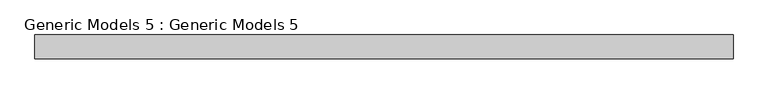
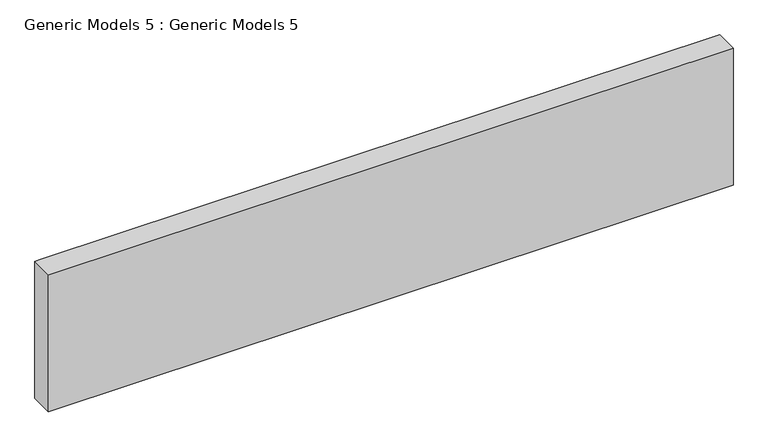
"""IFC4 building model written with IfcOpenShell, lengths in millimetres: proxy geometry, Generic Models 5 : Generic Models 5."""

from ifc_helpers import new_model, si_unit, origin, place, context, project, spatial, faceted_brep, source, transform, mapped, element, save


def generic_models_5_generic_models_5_9fe8e222(model_context):
    return source(origin(), model_context, "Body", "Brep", [
        faceted_brep([(-8586.8607234, -14006.5538163, 10395.767225), (-13013.8422243, -14006.5538163, 10395.767225), (-13059.291855, -14006.5538163, 10395.767225), (-13059.291855, -14158.9538163, 10395.767225), (-8586.8607234, -14158.9538163, 10395.767225), (-8586.8607234, -14006.5538163, 9448.8), (-8586.8607234, -14158.9538163, 9448.8), (-13059.291855, -14158.9538163, 9448.8), (-13059.291855, -14006.5538163, 9448.8), (-13013.8422243, -14006.5538163, 9448.8)], [[[0, 1, 2, 3, 4]], [[5, 6, 7, 8, 9]], [[2, 1, 0, 5, 9, 8]], [[3, 2, 8, 7]], [[4, 3, 7, 6]], [[0, 4, 6, 5]]]),
    ])


if __name__ == "__main__":
    model = new_model("IFC4")
    model_context = context("Model", 3, world=origin())
    ifc_project = project(units=[si_unit("LENGTHUNIT", "METRE", prefix="MILLI")], contexts=[model_context])
    site = spatial("IfcSite", under=ifc_project)
    building = spatial("IfcBuilding", under=site)
    placement = place(None, origin())
    generic_models_5_generic_models_5_shape = generic_models_5_generic_models_5_9fe8e222(model_context)
    element("IfcBuildingElementProxy", 1, Name="Generic Models 5 : Generic Models 5", ObjectType="Generic Models 5 : Generic Models 5", at=placement, inside=building, context=model_context, shape_type="MappedRepresentation", body=[
        mapped(generic_models_5_generic_models_5_shape, transform((0.0, 0.0, 0.0), x_axis=(1.0, 0.0, 0.0), y_axis=(0.0, 1.0, 0.0), z_axis=(0.0, 0.0, 1.0))),
    ])
    save(model, "model.ifc")
